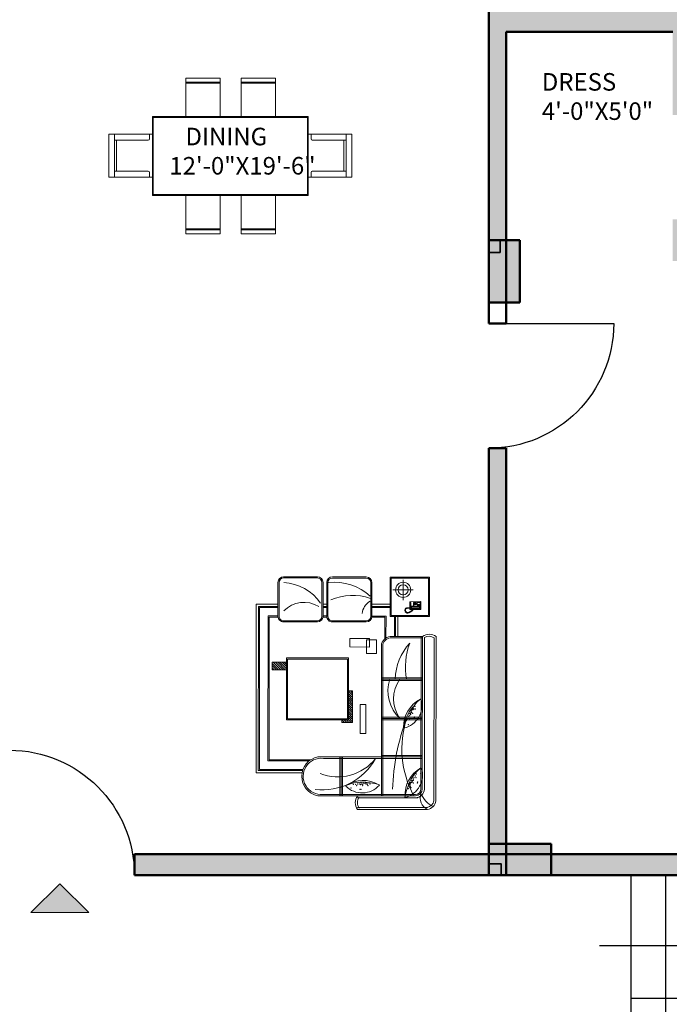
# Model space of a CAD drawing. Units: inches. Extents: x -7 to 1228, y -146 to 1091.
# Tile 82 of 88: x 816 to 1003, y 531 to 814. Entities that reach past the tile are written whole.
import ezdxf

# ---------------------------------------------------------------- set-up
doc = ezdxf.new("R2010")
doc.units = ezdxf.units.IN
for name, color, linetype, lineweight in [('A-ANNO-SYMB', 30, 'Continuous', 18), ('A-AREA-IDEN', 7, 'Continuous', 18), ('A-COLS', 6, 'Continuous', 35), ('A-DOOR', 4, 'Continuous', 25), ('A-FLOR-STRS', 1, 'Continuous', 25), ('A-FURN', 8, 'Continuous', 18), ('A-WALL', 7, 'Continuous', 50), ('A-WALL-PATT', 251, 'Continuous', 13)]:
    doc.layers.add(name, color=color, linetype=linetype, lineweight=lineweight)
doc.styles.get("Standard").update_dxf_attribs({"font": 'arial.ttf'})

# ---------------------------------------------------------------- blocks, each defined once
blk = doc.blocks.new('A$C317A697B')
for p, q in [((-116, 441), (-514, 441)), ((-514, 441), (-514, 0)), ((-116, 398), (-514, 398)), ((-116, 385), (-514, 385)), ((-116, 0), (-116, 441)), ((523, 441), (125, 441)), ((125, 441), (125, 0)), ((523, 398), (125, 398)), ((523, 385), (125, 385)), ((523, 0), (523, 441)), ((-899, -912), (-899, 0)), ((-899, 0), (899, 0)), ((899, 0), (899, -912)), ((-889, -902), (-889, -10)), ((-889, -10), (889, -10)), ((889, -10), (889, -902)), ((-899, -205), (-1402, -205)), ((-1402, -205), (-1402, -699)), ((-1336, -205), (-1336, -699)), ((-932, -205), (-932, -259)), ((899, -205), (1402, -205)), ((932, -205), (932, -259)), ((1336, -205), (1336, -699)), ((1402, -205), (1402, -699)), ((-946, -274), (-1336, -274)), ((-1311, -274), (-1311, -630)), ((946, -274), (1336, -274)), ((1311, -274), (1311, -630)), ((-946, -630), (-1336, -630)), ((-932, -699), (-932, -645)), ((932, -699), (932, -645)), ((946, -630), (1336, -630)), ((-1402, -699), (-899, -699)), ((1402, -699), (899, -699)), ((889, -902), (-889, -902)), ((899, -912), (-899, -912)), ((-514, -1353), (-514, -912)), ((-116, -912), (-116, -1353)), ((125, -1353), (125, -912)), ((523, -912), (523, -1353)), ((-116, -1297), (-514, -1297)), ((-116, -1309), (-514, -1309)), ((-116, -1353), (-514, -1353)), ((523, -1297), (125, -1297)), ((523, -1309), (125, -1309)), ((523, -1353), (125, -1353))]:
    blk.add_line(p, q)
for centre, start, end in [((-946, -259), 270, 0), ((946, -259), 180, 270), ((-946, -645), 0, 90), ((946, -645), 90, 180)]:
    blk.add_arc(centre, 14.7, start, end)
blk = doc.blocks.new('A$C327A19D4')
for p, q in [((1059, 3191), (3976, 3191)), ((1078, 3155), (3976, 3155)), ((703, 3073), (3, 3073)), ((3, 3073), (3, 2373)), ((683, 3053), (23, 3053)), ((23, 3053), (23, 2393)), ((683, 2393), (683, 3053)), ((703, 2373), (703, 3073)), ((1076, 2985), (3780, 2985)), ((4090, 3043), (4090, 1800)), ((4126, 3043), (4126, 1800)), ((1056, 2949), (3763, 2949)), ((1056, 2403), (1056, 2949)), ((1056, 2925), (3763, 2925)), ((1080, 2403), (1080, 2949)), ((1791, 2223), (1791, 2949)), ((1815, 2465), (1815, 2949)), ((1815, 2223), (1815, 2872)), ((1815, 2223), (1815, 2872)), ((1815, 2465), (1815, 2872)), ((1815, 2465), (1815, 2872)), ((1839, 2223), (1839, 2949)), ((2487, 2223), (2487, 2949)), ((2511, 2223), (2511, 2949)), ((2535, 2223), (2535, 2949)), ((3169, 2223), (3169, 2949)), ((3193, 2465), (3193, 2949)), ((3193, 2223), (3193, 2872)), ((3193, 2223), (3193, 2872)), ((3193, 2465), (3193, 2872)), ((3193, 2465), (3193, 2872)), ((3221, 1195), (3221, 2949)), ((3860, 2828), (3860, 1185)), ((3884, 2828), (3884, 1095)), ((3920, 2867), (3920, 1802)), ((231, 2784), (227, 2425)), ((49, 2607), (409, 2603)), ((703, 2512), (1056, 2512)), ((703, 2472), (1056, 2472)), ((703, 2452), (1056, 2452)), ((3, 2373), (703, 2373)), ((23, 2393), (683, 2393)), ((484, 2052), (484, 2373)), ((524, 2052), (524, 2373)), ((544, 2052), (544, 2373)), ((694, 2052), (694, 2302)), ((694, 2302), (1084, 2302)), ((714, 2051), (714, 2282)), ((714, 2282), (1098, 2282)), ((1119, 2135), (1357, 2135)), ((1119, 1958), (1119, 2135)), ((3884, 2247), (1184, 2247)), ((3884, 2223), (1184, 2223)), ((1357, 2135), (1357, 1958)), ((3195, 2235), (3195, 1095)), ((1092, 2007), (1244, 2007)), ((1092, 1659), (1092, 2007)), ((1357, 1958), (1119, 1958)), ((1244, 2007), (1244, 1659)), ((2265, 1945), (2780, 1945)), ((2265, 1845), (2265, 1945)), ((2780, 1945), (2780, 1845)), ((2780, 1845), (2265, 1845)), ((1244, 1659), (1092, 1659)), ((2539, 1638), (1439, 1638)), ((1439, 1638), (1439, 538)), ((2519, 1618), (1459, 1618)), ((1459, 1618), (1459, 558)), ((2023, 1638), (2023, 1711)), ((2023, 1711), (2585, 1711)), ((2519, 558), (2519, 1618)), ((2539, 538), (2539, 1638)), ((2585, 1711), (2585, 1522)), ((2585, 1522), (2539, 1522)), ((3884, 1532), (3195, 1532)), ((3884, 1508), (3195, 1508)), ((3884, 1484), (3195, 1484)), ((484, 1185), (484, 1252)), ((524, 1185), (524, 1252)), ((544, 1185), (544, 1252)), ((694, 1185), (694, 1252)), ((714, 1184), (714, 1253)), ((3247, 967), (3247, 230)), ((3267, 940), (3267, 210)), ((3417, 832), (3417, 60)), ((3437, 825), (3437, 40)), ((3477, 816), (3477, 0)), ((1439, 538), (2539, 538)), ((1459, 558), (2519, 558)), ((1516, 538), (1651, 538)), ((1516, 285), (1516, 538)), ((1651, 538), (1651, 285)), ((484, 0), (484, 385)), ((524, 40), (524, 385)), ((544, 60), (544, 385)), ((694, 210), (694, 385)), ((714, 230), (714, 386)), ((3267, 210), (694, 210)), ((3247, 230), (714, 230)), ((1651, 285), (1516, 285)), ((3437, 40), (524, 40)), ((3417, 60), (544, 60)), ((3477, 0), (484, 0))]:
    blk.add_line(p, q)
at = {"linetype": 'ByBlock'}
for p, q in [((438, 2915), (440, 2918)), ((439, 2728), (438, 2915)), ((440, 2918), (576, 2919)), ((451, 2906), (490, 2906)), ((451, 2856), (451, 2906)), ((491, 2856), (451, 2856)), ((453, 2831), (453, 2839)), ((453, 2839), (461, 2839)), ((461, 2831), (453, 2831)), ((453, 2824), (461, 2825)), ((453, 2816), (453, 2824)), ((461, 2816), (453, 2816)), ((453, 2801), (453, 2810)), ((453, 2810), (461, 2810)), ((461, 2802), (453, 2801)), ((461, 2839), (461, 2831)), ((461, 2825), (461, 2816)), ((461, 2810), (461, 2802)), ((466, 2839), (475, 2840)), ((467, 2831), (466, 2839)), ((475, 2831), (467, 2831)), ((467, 2816), (467, 2825)), ((467, 2825), (475, 2825)), ((475, 2817), (467, 2816)), ((467, 2802), (467, 2810)), ((467, 2810), (475, 2810)), ((475, 2802), (467, 2802)), ((475, 2840), (475, 2831)), ((475, 2825), (475, 2817)), ((475, 2810), (475, 2802)), ((480, 2840), (488, 2840)), ((480, 2831), (480, 2840)), ((488, 2832), (480, 2831)), ((480, 2817), (480, 2825)), ((480, 2825), (488, 2825)), ((488, 2817), (480, 2817)), ((480, 2810), (488, 2810)), ((480, 2802), (480, 2810)), ((488, 2802), (480, 2802)), ((488, 2840), (488, 2832)), ((488, 2825), (488, 2817)), ((488, 2810), (488, 2802)), ((490, 2906), (491, 2856)), ((505, 2903), (494, 2903)), ((494, 2903), (494, 2899)), ((494, 2899), (505, 2899)), ((495, 2895), (495, 2891)), ((505, 2895), (495, 2895)), ((495, 2891), (505, 2891)), ((495, 2887), (495, 2883)), ((505, 2887), (495, 2887)), ((495, 2883), (505, 2883)), ((495, 2879), (495, 2875)), ((505, 2879), (495, 2879)), ((495, 2875), (505, 2875)), ((495, 2871), (495, 2867)), ((506, 2871), (495, 2871)), ((495, 2867), (506, 2867)), ((495, 2863), (495, 2859)), ((506, 2863), (495, 2863)), ((495, 2859), (506, 2859)), ((505, 2899), (505, 2903)), ((505, 2891), (505, 2895)), ((505, 2883), (505, 2887)), ((505, 2875), (505, 2879)), ((506, 2867), (506, 2871)), ((506, 2859), (506, 2863)), ((515, 2908), (520, 2914)), ((516, 2744), (515, 2908)), ((520, 2910), (519, 2905)), ((519, 2905), (531, 2893)), ((519, 2905), (519, 2868)), ((519, 2868), (522, 2862)), ((520, 2914), (561, 2915)), ((526, 2913), (520, 2910)), ((522, 2862), (526, 2855)), ((522, 2790), (526, 2797)), ((532, 2895), (526, 2913)), ((526, 2913), (558, 2913)), ((526, 2855), (527, 2845)), ((526, 2797), (528, 2806)), ((527, 2845), (527, 2832)), ((528, 2806), (527, 2832)), ((531, 2893), (532, 2895)), ((532, 2832), (531, 2893)), ((551, 2896), (532, 2895)), ((532, 2832), (532, 2759)), ((551, 2896), (558, 2913)), ((553, 2893), (551, 2896)), ((565, 2905), (553, 2893)), ((553, 2832), (553, 2893)), ((553, 2832), (554, 2759)), ((558, 2855), (557, 2846)), ((557, 2846), (557, 2832)), ((557, 2806), (557, 2832)), ((559, 2797), (557, 2806)), ((558, 2913), (563, 2911)), ((562, 2862), (558, 2855)), ((563, 2790), (559, 2797)), ((561, 2915), (568, 2908)), ((565, 2869), (562, 2862)), ((563, 2911), (565, 2905)), ((565, 2905), (565, 2869)), ((568, 2908), (569, 2745)), ((576, 2919), (578, 2916)), ((578, 2916), (580, 2729)), ((442, 2726), (439, 2728)), ((543, 2726), (442, 2726)), ((453, 2787), (453, 2795)), ((453, 2795), (461, 2795)), ((461, 2787), (453, 2787)), ((468, 2743), (455, 2743)), ((455, 2743), (455, 2735)), ((455, 2735), (469, 2735)), ((461, 2795), (461, 2787)), ((467, 2787), (467, 2795)), ((467, 2795), (475, 2795)), ((475, 2787), (467, 2787)), ((469, 2735), (468, 2743)), ((487, 2743), (474, 2743)), ((474, 2743), (474, 2735)), ((474, 2735), (487, 2735)), ((475, 2795), (475, 2787)), ((480, 2787), (480, 2795)), ((480, 2795), (488, 2795)), ((488, 2787), (480, 2787)), ((487, 2735), (487, 2743)), ((488, 2795), (488, 2787)), ((493, 2744), (493, 2735)), ((506, 2744), (493, 2744)), ((493, 2735), (506, 2735)), ((497, 2795), (507, 2795)), ((497, 2787), (497, 2795)), ((507, 2787), (497, 2787)), ((506, 2735), (506, 2744)), ((507, 2795), (507, 2787)), ((523, 2737), (516, 2744)), ((520, 2783), (522, 2790)), ((520, 2746), (520, 2783)), ((520, 2746), (532, 2759)), ((521, 2741), (520, 2746)), ((527, 2738), (521, 2741)), ((542, 2737), (523, 2737)), ((533, 2756), (527, 2738)), ((527, 2738), (542, 2738)), ((532, 2759), (533, 2756)), ((552, 2756), (533, 2756)), ((546, 2743), (542, 2743)), ((542, 2743), (542, 2731)), ((542, 2731), (545, 2717)), ((545, 2717), (549, 2704)), ((547, 2732), (546, 2743)), ((546, 2738), (559, 2739)), ((562, 2737), (546, 2737)), ((549, 2696), (546, 2692)), ((546, 2692), (546, 2686)), ((546, 2686), (554, 2685)), ((554, 2685), (546, 2680)), ((546, 2680), (547, 2672)), ((548, 2723), (547, 2732)), ((547, 2672), (555, 2672)), ((577, 2726), (548, 2726)), ((552, 2710), (548, 2723)), ((549, 2704), (548, 2697)), ((548, 2697), (549, 2696)), ((555, 2672), (548, 2666)), ((548, 2666), (551, 2659)), ((551, 2659), (560, 2661)), ((554, 2759), (552, 2756)), ((552, 2756), (559, 2739)), ((553, 2703), (552, 2710)), ((552, 2696), (553, 2703)), ((557, 2693), (552, 2696)), ((566, 2747), (554, 2759)), ((556, 2687), (557, 2693)), ((558, 2669), (556, 2687)), ((560, 2661), (556, 2653)), ((556, 2653), (560, 2648)), ((568, 2656), (558, 2669)), ((559, 2739), (565, 2741)), ((560, 2648), (566, 2653)), ((569, 2745), (562, 2737)), ((566, 2783), (563, 2790)), ((565, 2741), (566, 2747)), ((566, 2653), (565, 2646)), ((565, 2646), (570, 2642)), ((566, 2747), (566, 2783)), ((583, 2649), (568, 2656)), ((570, 2642), (577, 2648)), ((577, 2648), (576, 2639)), ((576, 2639), (582, 2637)), ((580, 2729), (577, 2726)), ((587, 2779), (579, 2779)), ((579, 2775), (584, 2774)), ((582, 2637), (585, 2645)), ((599, 2647), (583, 2649)), ((584, 2774), (587, 2772)), ((585, 2645), (589, 2637)), ((590, 2777), (587, 2779)), ((587, 2772), (591, 2770)), ((589, 2637), (593, 2637)), ((594, 2771), (590, 2777)), ((591, 2770), (593, 2768)), ((595, 2768), (592, 2765)), ((592, 2765), (597, 2757)), ((593, 2768), (595, 2768)), ((593, 2637), (595, 2645)), ((599, 2771), (594, 2771)), ((595, 2645), (598, 2636)), ((597, 2757), (606, 2742)), ((598, 2636), (604, 2637)), ((602, 2770), (599, 2771)), ((599, 2760), (603, 2767)), ((606, 2763), (599, 2760)), ((615, 2654), (599, 2647)), ((603, 2767), (602, 2770)), ((604, 2750), (608, 2758)), ((612, 2753), (604, 2750)), ((604, 2645), (610, 2639)), ((604, 2637), (604, 2645)), ((608, 2758), (606, 2763)), ((606, 2742), (612, 2731)), ((608, 2742), (614, 2749)), ((615, 2746), (608, 2742)), ((610, 2639), (615, 2642)), ((614, 2749), (612, 2753)), ((612, 2731), (614, 2730)), ((613, 2733), (618, 2740)), ((621, 2736), (613, 2733)), ((614, 2730), (613, 2728)), ((613, 2728), (622, 2712)), ((614, 2650), (619, 2643)), ((615, 2642), (614, 2650)), ((618, 2740), (615, 2746)), ((627, 2666), (615, 2654)), ((619, 2643), (624, 2647)), ((620, 2723), (624, 2730)), ((627, 2725), (620, 2723)), ((620, 2654), (628, 2651)), ((624, 2647), (620, 2654)), ((624, 2730), (621, 2736)), ((622, 2712), (631, 2687)), ((626, 2712), (630, 2720)), ((634, 2713), (626, 2712)), ((630, 2720), (627, 2725)), ((631, 2687), (627, 2666)), ((628, 2702), (636, 2705)), ((637, 2702), (628, 2702)), ((628, 2661), (636, 2659)), ((632, 2654), (628, 2661)), ((628, 2651), (632, 2654)), ((631, 2672), (640, 2672)), ((638, 2665), (631, 2672)), ((633, 2691), (639, 2696)), ((641, 2691), (633, 2691)), ((636, 2705), (634, 2713)), ((634, 2681), (642, 2684)), ((641, 2677), (634, 2681)), ((636, 2659), (638, 2665)), ((639, 2696), (637, 2702)), ((640, 2672), (641, 2677)), ((642, 2684), (641, 2691))]:
    blk.add_line(p, q, dxfattribs=at)
at = {"ltscale": 5}
for p, q in [((0, 1352), (0, 1952)), ((20, 1352), (20, 1952)), ((100, 2052), (700, 2052)), ((100, 2032), (700, 2032)), ((780, 1952), (780, 1352)), ((800, 1952), (800, 1352)), ((2023, 1673), (2061, 1711)), ((2027, 1638), (2100, 1711)), ((2067, 1638), (2139, 1711)), ((2106, 1638), (2179, 1711)), ((2145, 1638), (2218, 1711)), ((2184, 1638), (2257, 1711)), ((2224, 1638), (2296, 1711)), ((2263, 1638), (2336, 1711)), ((2302, 1638), (2375, 1711)), ((2341, 1638), (2414, 1711)), ((2381, 1638), (2453, 1711)), ((2420, 1638), (2493, 1711)), ((2459, 1638), (2532, 1711)), ((2498, 1638), (2571, 1711)), ((2538, 1638), (2585, 1685)), ((2539, 1601), (2585, 1646)), ((2539, 1561), (2585, 1607)), ((2539, 1522), (2585, 1568)), ((2578, 1522), (2585, 1528)), ((700, 1272), (100, 1272)), ((700, 1252), (100, 1252)), ((0, 485), (0, 1085)), ((20, 485), (20, 1085)), ((100, 1185), (700, 1185)), ((100, 1165), (700, 1165)), ((780, 1085), (780, 485)), ((800, 1085), (800, 485)), ((1516, 499), (1555, 538)), ((1516, 460), (1594, 538)), ((1516, 421), (1634, 538)), ((700, 405), (100, 405)), ((700, 385), (100, 385)), ((1516, 382), (1651, 516)), ((1516, 342), (1651, 477)), ((1516, 303), (1651, 438)), ((1537, 285), (1651, 398)), ((1576, 285), (1651, 359)), ((1616, 285), (1651, 320))]:
    blk.add_line(p, q, dxfattribs=at)
for radius in [134, 88.7]:
    blk.add_circle((229, 2605), radius)
for centre, radius, start, end in [((1218, 3068), 201, 142.4201, 216.3682), ((1218, 3068), 165, 148.4003, 210.2229), ((3943, 3007), 150, 10.9855, 79.893), ((3943, 3007), 187, 10.9855, 79.893), ((3763, 2828), 157, 0, 90), ((3657, 3353), 468, 293.6733, 332.9672), ((3921, 3138), 226, 250.4844, 335.1673), ((2545, 3192), 468, 214.7097, 257.8799), ((2283, 2531), 409, 13.4523, 105.9639), ((2657, 3163), 547, 207.1715, 271.8037), ((3869, 3188), 547, 208.8478, 273.48), ((3911, 3323), 657, 217.6007, 253.5739), ((3517, 2544), 409, 14.6876, 107.1992), ((3763, 2828), 121, 0, 90), ((3763, 2828), 96.8, 0, 90), ((1594, 3859), 1211, 249.7283, 280.5443), ((1853, 3485), 1021, 228.2765, 267.8541), ((2752, 3267), 657, 227.0776, 263.0508), ((3052, 4350), 1764, 252.1519, 298.1592), ((3865, 6197), 3777, 248.9971, 268.5461), ((3951, 3106), 468, 222.7716, 265.9418), ((2024, 3008), 670, 251.8392, 316.629), ((2163, 3036), 599, 234.5154, 305.4846), ((1243, 2401), 187, 179.2584, 251.6848), ((1243, 2401), 163, 179.2584, 251.6848), ((4159, 1898), 547, 149.1529, 213.7851), ((4124, 2008), 468, 156.691, 199.8613), ((3425, 1881), 409, 315.4337, 47.9453), ((4298, 1873), 657, 169.059, 205.0321), ((4007, 1962), 201, 232.4201, 306.3682), ((4007, 1962), 165, 232.4201, 306.3682)]:
    blk.add_arc(centre, radius, start, end)
at = {"ltscale": 20}
for centre, radius, start, end in [((2701, 1449), 849, 338.2682, 52.2695), ((2703, 1175), 1078, 353.1988, 61.2564), ((3540, 1161), 351, 190.8398, 349.1602), ((3540, 1156), 321, 172.9078, 5.2194)]:
    blk.add_arc(centre, radius, start, end, dxfattribs=at)
at = {"ltscale": 5}
for centre, radius, start, end in [((100, 1952), 100, 90, 180), ((100, 1952), 80, 90, 180), ((1024, 1388), 928, 137.1341, 186.5635), ((1307, 1706), 979, 160.9364, 203.1944), ((676, 2156), 279, 209.1633, 264.4137), ((700, 1952), 100, 0, 90), ((700, 1952), 80, 0, 90), ((100, 1352), 100, 180, 270), ((100, 1352), 80, 180, 270), ((700, 1352), 80, 270, 0), ((700, 1352), 100, 270, 0), ((100, 1085), 100, 90, 180), ((100, 1085), 80, 90, 180), ((968, 436), 868, 125.4807, 176.5616), ((949, 846), 497, 147.8484, 226.1244), ((700, 1085), 100, 0, 90), ((700, 1085), 80, 0, 90), ((100, 485), 100, 180, 270), ((100, 485), 80, 180, 270), ((700, 485), 100, 270, 0), ((700, 485), 80, 270, 0)]:
    blk.add_arc(centre, radius, start, end, dxfattribs=at)
for p in [(2298, 2818), (2344, 2802), (2345, 2825), (2485, 2814), (2498, 2803), (3492, 2920), (3495, 2842), (3535, 2825), (3560, 2838), (3561, 2800), (3641, 2868), (3657, 2862), (2329, 2780), (2356, 2781), (2375, 2736), (2410, 2757), (2421, 2774), (2421, 2720), (2444, 2738), (2445, 2691), (2459, 2715), (2481, 2700), (2514, 2718), (2515, 2690), (2551, 2664), (2620, 2701), (3571, 2765), (3585, 2789), (3609, 2758), (3612, 2788), (3646, 2728), (3647, 2768), (3655, 2787), (3694, 2735), (3707, 2710), (3719, 2734), (3738, 2747), (3756, 2703), (3660, 1974), (3676, 1951), (3677, 2020), (3687, 1973), (3707, 1984), (3646, 1828), (3648, 1911), (3658, 1864), (3673, 1803), (3674, 1829), (3683, 1768), (3684, 1893), (3686, 1853), (3705, 1892), (3706, 1784), (3770, 1842), (3772, 1859), (3680, 1724), (3748, 1685)]:
    blk.add_point(p)
blk = doc.blocks.new('DOOR-900')
blk.add_line((36, 0), (36, 36))
blk.add_arc((36, 0), 36, 90, 180)

msp = doc.modelspace()

# ---------------------------------------------------------------- hatches: boundary and pattern name
at = {"layer": 'A-ANNO-SYMB'}
h = msp.add_hatch(color=256, dxfattribs=at)
h.dxf.hatch_style = 1
h.paths.add_polyline_path([(827.53, 565.53), (819.19, 557.2), (835.87, 557.2)])
at = {"layer": 'A-COLS'}
h = msp.add_hatch(color=256, dxfattribs=at)
h.dxf.hatch_style = 1
h.paths.add_polyline_path([(951, 733), (960, 733), (960, 751), (954.29, 751), (954.29, 747.45), (951, 747.45)])
h = msp.add_hatch(color=256, dxfattribs=at)
h.dxf.hatch_style = 1
h.paths.add_polyline_path([(954.29, 747.45), (954.29, 751), (951, 751), (951, 747.45)])
h = msp.add_hatch(color=256, dxfattribs=at)
h.dxf.hatch_style = 1
h.paths.add_polyline_path([(969, 568), (969, 577), (951, 577), (951, 571.29), (954.55, 571.29), (954.55, 568)])
h = msp.add_hatch(color=256, dxfattribs=at)
h.dxf.hatch_style = 1
h.paths.add_polyline_path([(954.55, 571.29), (951, 571.29), (951, 568), (954.55, 568)])
at = {"layer": 'A-WALL-PATT'}
h = msp.add_hatch(color=256, dxfattribs=at)
h.dxf.hatch_style = 1
h.paths.add_polyline_path([(69, 568), (60, 568), (60, 493), (63.29, 493), (69, 493)])
h.paths.add_polyline_path([(69, 662.41), (60, 662.41), (60, 586), (69, 586)], flags=17)
h.paths.add_polyline_path([(69, 723), (184, 723), (184, 734), (179, 734), (179, 728), (69, 728), (69, 741.62), (60, 741.62), (60, 698.41), (69, 698.41)], flags=17)
h.paths.add_polyline_path([(69, 782), (231, 782), (231, 728), (231, 723), (231, 586), (236, 586), (236, 787), (69, 787), (69, 800.13), (60, 800.13), (60, 765.62), (69, 765.62)])
h.paths.add_polyline_path([(184, 842), (189, 842), (189, 848), (173, 848), (173, 842), (179, 842), (179, 787), (184, 787)])
h.paths.add_polyline_path([(118.22, 69), (69, 69), (69, 60), (118.22, 60)])
h.paths.add_polyline_path([(227, 69), (154.22, 69), (154.22, 60), (227, 60)])
h.paths.add_polyline_path([(236, 60), (232.71, 60), (227, 60), (227, 36), (236, 36)])
h.paths.add_polyline_path([(389, 60), (380, 60), (380, 36), (389, 36)])
h.paths.add_polyline_path([(384, 181), (380, 181), (380, 115), (380, 78), (384, 78)])
h.paths.add_polyline_path([(380, 115), (334.55, 115), (334.55, 109), (380, 109)])
h.paths.add_polyline_path([(274.55, 115), (236, 115), (236, 201), (232.71, 201), (231, 201), (231, 78), (236, 78), (236, 109), (274.55, 109)])
h.paths.add_polyline_path([(69, 123), (60, 123), (60, 78), (69, 78)])
h.paths.add_polyline_path([(69, 201), (60, 201), (60, 159), (69, 159)])
h.paths.add_polyline_path([(143, 219), (69, 219), (69, 213), (143, 213)], flags=17)
h.paths.add_polyline_path([(189, 219), (184, 219), (184, 274), (231, 274), (231, 219), (236, 219), (236, 279), (184, 279), (184, 297), (179, 297), (179, 279), (69, 279), (69, 290.91), (60, 290.91), (60, 262.18), (69, 262.18), (69, 274), (179, 274), (179, 219), (173, 219), (173, 213), (189, 213)])
h.paths.add_polyline_path([(69, 238.18), (60, 238.18), (60, 219), (69, 219)], flags=17)
h.paths.add_polyline_path([(69, 333), (60, 333), (60, 314.91), (69, 314.91), (69, 316.96)])
h.paths.add_polyline_path([(190, 338), (184, 338), (69, 338), (69, 333), (179, 333), (179, 327), (184, 327), (184, 333.02), (190, 333.05)])
h.paths.add_polyline_path([(69, 386.81), (60, 386.81), (60, 351), (69, 351)])
h.paths.add_polyline_path([(69, 475), (60, 475), (60, 422.81), (69, 422.81)])
h.paths.add_polyline_path([(236, 475), (231, 475), (231, 351.24), (236, 351.24)])
h.paths.add_polyline_path([(384, 475), (380, 475), (380, 362), (384, 362)])
h.paths.add_polyline_path([(547, 307), (439, 307), (439, 356), (445, 356), (445, 362), (433, 362), (433, 307), (380, 307), (380, 244), (380, 241), (384, 241), (384, 301), (433, 301), (433, 277), (439, 277), (439, 301), (547, 301)])
h.paths.add_polyline_path([(547, 241), (439, 241), (439, 247), (433, 247), (433, 235), (547, 235)])
h.paths.add_polyline_path([(450, 69), (440.29, 69), (424.89, 69), (389, 69), (389, 60), (450, 60)])
h.paths.add_polyline_path([(547, 69), (486, 69), (486, 60), (547, 60)])
h.paths.add_polyline_path([(556, 148.27), (547, 148.27), (547, 78), (556, 78)])
h.paths.add_polyline_path([(556, 223), (547, 223), (547, 195), (547, 184.27), (556, 184.27)])
h.paths.add_polyline_path([(556, 311.19), (547, 311.19), (547, 273.08), (556, 273.08)])
h.paths.add_polyline_path([(556, 344), (552.71, 344), (547, 344), (547, 335.19), (556, 335.19)])
h.paths.add_polyline_path([(556, 249.08), (547, 249.08), (547, 241), (556, 241)])
h.paths.add_polyline_path([(547, 362), (475, 362), (475, 356), (547, 356)], flags=0)
h.paths.add_polyline_path([(556, 399.62), (547, 399.62), (547, 362), (556, 362)])
h.paths.add_polyline_path([(556, 475), (547, 475), (547, 435.62), (556, 435.62)])
h.paths.add_polyline_path([(547, 493), (389, 493), (389, 487), (547, 487)])
h.paths.add_polyline_path([(380, 493), (278, 493), (278, 487), (380, 487)])
h.paths.add_polyline_path([(227, 493), (69, 493), (69, 487), (227, 487)])
h.paths.add_polyline_path([(643, 122.44), (634, 122.44), (634, 78), (643, 78)])
h.paths.add_polyline_path([(702.5, 69), (692.79, 69), (677.39, 69), (643, 69), (643, 60), (702.5, 60)])
h.paths.add_polyline_path([(798, 69), (738.5, 69), (738.5, 60), (798, 60)])
h.paths.add_polyline_path([(807, 60), (803.71, 60), (798, 60), (798, 36), (807, 36)])
h.paths.add_polyline_path([(807, 109), (846.75, 109), (846.75, 115), (807, 115), (807, 159), (802, 159), (802, 78), (807, 78)])
h.paths.add_polyline_path([(807, 201), (802, 201), (802, 195), (807, 195)])
h.paths.add_polyline_path([(643, 201), (634, 201), (634, 158.44), (643, 158.44)])
h.paths.add_polyline_path([(756, 225), (751, 225), (751, 219), (643, 219), (643, 213), (756, 213)])
h.paths.add_polyline_path([(643, 240.85), (634, 240.85), (634, 219), (643, 219)])
h.paths.add_polyline_path([(643, 274), (643, 288.63), (634, 288.63), (634, 264.85), (643, 264.85)])
h.paths.add_polyline_path([(802, 279), (756, 279), (756, 297), (751, 297), (751, 279), (643, 279), (643, 274), (751, 274), (751, 255), (756, 255), (756, 274), (802, 274)])
h.paths.add_polyline_path([(807, 333), (803.71, 333), (802, 333), (802, 279), (802, 274), (802, 219), (807, 219)])
h.paths.add_polyline_path([(956, 182), (951, 182), (951, 115), (906.75, 115), (906.75, 109), (951, 109), (951, 78), (956, 78)])
h.paths.add_polyline_path([(960, 60), (951, 60), (951, 36), (960, 36)])
h.paths.add_polyline_path([(1021, 69), (1005.78, 69), (960, 69), (960, 60), (1021, 60)])
h.paths.add_polyline_path([(956, 224), (951, 224), (951, 218), (956, 218)])
h.paths.add_polyline_path([(956, 302), (1004, 302), (1004, 278), (1010, 278), (1010, 302), (1118, 302), (1118, 290.81), (1127, 290.81), (1127, 326.97), (1118, 326.97), (1118, 320.97), (1118, 307), (1010, 307), (1010, 356), (1016, 356), (1016, 362), (1004, 362), (1004, 307), (951, 307), (951, 244), (951, 242), (954.29, 242), (956, 242)])
h.paths.add_polyline_path([(643, 333), (634, 333), (634, 312.63), (643, 312.63), (643, 316.96)])
h.paths.add_polyline_path([(756, 338), (643, 338), (643, 333), (751, 333), (751, 327), (756, 327)])
h.paths.add_polyline_path([(643, 388), (634, 388), (634, 351), (643, 351)])
h.paths.add_polyline_path([(807, 357), (802, 357), (802, 351), (807, 351)])
h.paths.add_polyline_path([(807, 475), (802, 475), (802, 393), (807, 393)])
h.paths.add_polyline_path([(643, 475), (634, 475), (634, 424), (643, 424)])
h.paths.add_polyline_path([(798, 493), (643, 493), (643, 487), (798, 487)])
h.paths.add_polyline_path([(634, 493), (556, 493), (556, 487), (634, 487)])
h.paths.add_polyline_path([(813, 493), (807, 493), (807, 487), (813, 487)])
h.paths.add_polyline_path([(951, 493), (849, 493), (849, 487), (951, 487)])
h.paths.add_polyline_path([(956, 484), (951, 484), (951, 374), (956, 374)])
h.paths.add_polyline_path([(1109, 493), (969, 493), (969, 487), (1109, 487)])
h.paths.add_polyline_path([(1127, 484), (1118, 484), (1118, 450.64), (1127, 450.64)])
h.paths.add_polyline_path([(1127, 414.64), (1118, 414.64), (1118, 365), (1127, 365)])
h.paths.add_polyline_path([(1109, 362), (1046, 362), (1046, 356), (1109, 356)], flags=17)
h.paths.add_polyline_path([(1127, 356), (1123.45, 356), (1118, 356), (1118, 350.97), (1127, 350.97)], flags=0)
h.paths.add_polyline_path([(1127, 266.81), (1118, 266.81), (1118, 262.36), (1118, 242), (1127, 242)], flags=17)
h.paths.add_polyline_path([(1118, 242), (1010, 242), (1010, 248), (1004, 248), (1004, 237), (1118, 237)])
h.paths.add_polyline_path([(1127, 224), (1118, 224), (1118, 170), (1127, 170)])
h.paths.add_polyline_path([(1127, 134), (1118, 134), (1118, 78), (1127, 78)])
h.paths.add_polyline_path([(1118, 69), (1057, 69), (1057, 60), (1118, 60)])
h.paths.add_polyline_path([(227, 571.55), (227, 574), (69, 574), (69, 568), (227, 568)])
h.paths.add_polyline_path([(380, 571.55), (380, 574), (278, 574), (278, 568), (380, 568)])
h.paths.add_polyline_path([(242, 574), (236, 574), (236, 568), (242, 568)])
h.paths.add_polyline_path([(547, 571.55), (547, 574), (389, 574), (389, 568), (547, 568)])
h.paths.add_polyline_path([(384, 733), (380, 733), (380, 586), (384, 586)])
h.paths.add_polyline_path([(556, 646), (634, 646), (634, 655), (547, 655), (547, 586), (556, 586)])
h.paths.add_polyline_path([(634, 574), (556, 574), (556, 568), (634, 568)])
h.paths.add_polyline_path([(643, 655), (634, 655), (634, 586), (643, 586)])
h.paths.add_polyline_path([(798, 574), (643, 574), (643, 568), (798, 568)])
h.paths.add_polyline_path([(643, 663.85), (634, 663.85), (634, 655), (643, 655)])
h.paths.add_polyline_path([(556, 676.97), (547, 676.97), (547, 655), (556, 655)])
h.paths.add_polyline_path([(556, 733), (547, 733), (547, 712.97), (556, 712.97)])
h.paths.add_polyline_path([(643, 710), (634, 710), (634, 699.85), (643, 699.85)])
h.paths.add_polyline_path([(807, 668), (802, 668), (802, 586), (807, 586)])
h.paths.add_polyline_path([(951, 574), (849, 574), (849, 568), (951, 568)])
h.paths.add_polyline_path([(956, 691), (951, 691), (951, 577), (956, 577)])
h.paths.add_polyline_path([(1109, 574), (969, 574), (969, 568), (1109, 568)])
h.paths.add_polyline_path([(1127, 643.4), (1118, 643.4), (1118, 577), (1127, 577)])
h.paths.add_polyline_path([(1127, 568), (1123.45, 568), (1118, 568), (1118, 493), (1127, 493)])
h.paths.add_polyline_path([(1127, 733), (1118, 733), (1118, 679.4), (1127, 679.4)])
h.paths.add_polyline_path([(1127, 777.35), (1118, 777.35), (1118, 770.04), (1118, 751), (1127, 751)], flags=17)
h.paths.add_polyline_path([(1118, 751), (1010, 751), (1010, 757), (1004, 757), (1004, 745), (1118, 745)])
h.paths.add_polyline_path([(956, 811), (1004, 811), (1004, 787), (1010, 787), (1010, 811), (1017.87, 811), (1017.87, 811.63, -0.414214), (1018.25, 812), (1031.98, 812, -0.414214), (1032.35, 811.63), (1032.35, 811), (1118, 811), (1118, 801.35), (1127, 801.35), (1127, 834.69), (1118, 834.69), (1118, 830.24), (1118, 817), (1010, 817), (1010, 866), (1016, 866), (1016, 872), (1004, 872), (1004, 817), (956, 817), (956, 866), (951, 866), (951, 751), (954.29, 751), (956, 751)])
h.paths.add_polyline_path([(1118, 872), (1046, 872), (1046, 866), (1118, 866)], flags=17)
h.paths.add_polyline_path([(1127, 924.71), (1118, 924.71), (1118, 884), (1127, 884)])
h.paths.add_polyline_path([(1127, 866), (1123.71, 866), (1118, 866), (1118, 858.69), (1127, 858.69)], flags=17)
h.paths.add_polyline_path([(956, 983), (951, 983), (951, 952), (807, 952), (807, 983), (802, 983), (802, 902), (807, 902), (807, 946), (951, 946), (951, 884), (956, 884)])
h.paths.add_polyline_path([(807, 842), (802, 842), (802, 787), (756, 787), (756, 806), (751, 806), (751, 787), (643, 787), (643, 782), (751, 782), (751, 764), (756, 764), (756, 782), (802, 782), (802, 728), (807, 728)])
h.paths.add_polyline_path([(756, 848), (643, 848), (643, 842), (751, 842), (751, 836), (756, 836)])
h.paths.add_polyline_path([(756, 734), (751, 734), (751, 728), (643, 728), (643, 723), (756, 723)])
h.paths.add_polyline_path([(643, 749.79), (634, 749.79), (634, 728), (637.29, 728), (643, 728)])
h.paths.add_polyline_path([(643, 805.41), (634, 805.41), (634, 773.79), (643, 773.79)])
h.paths.add_polyline_path([(643, 896.66), (634, 896.66), (634, 860), (637.29, 860), (643, 860)])
h.paths.add_polyline_path([(643, 842), (634, 842), (634, 829.41), (643, 829.41)])
h.paths.add_polyline_path([(643, 983), (634, 983), (634, 932.66), (643, 932.66)])
h.paths.add_polyline_path([(1127, 983), (1118, 983), (1118, 960.71), (1127, 960.71)])
h.paths.add_polyline_path([(1118, 1001), (1077.53, 1001), (1077.53, 992), (1118, 992)])
h.paths.add_polyline_path([(1041.53, 1001), (960, 1001), (960, 992), (1041.53, 992)])
h.paths.add_polyline_path([(960, 1025), (951, 1025), (951, 1001), (954.29, 1001), (960, 1001)])
h.paths.add_polyline_path([(807, 1025), (798, 1025), (798, 1001), (807, 1001)])
h.paths.add_polyline_path([(798, 1001), (738.5, 1001), (738.5, 992), (798, 992)])
h.paths.add_polyline_path([(702.5, 1001), (643, 1001), (643, 992), (702.5, 992)])
h.paths.add_polyline_path([(547, 1001), (499.11, 1001), (499.11, 992), (547, 992)])
h.paths.add_polyline_path([(463.11, 1001), (389, 1001), (389, 992), (463.11, 992)])
h.paths.add_polyline_path([(389, 1025), (380, 1025), (380, 1022), (380, 1001), (383.29, 1001), (389, 1001)])
h.paths.add_polyline_path([(236, 1025), (227, 1025), (227, 1001), (236, 1001)])
h.paths.add_polyline_path([(236, 983), (231, 983), (231, 860), (236, 860)])
h.paths.add_polyline_path([(274.55, 952), (236, 952), (236, 946), (274.55, 946)])
h.paths.add_polyline_path([(380, 952), (334.55, 952), (334.55, 946), (380, 946)])
h.paths.add_polyline_path([(384, 983), (380, 983), (380, 884), (383.29, 884), (384, 884)])
h.paths.add_polyline_path([(227, 1001), (155.01, 1001), (155.01, 992), (162.87, 992), (227, 992)])
h.paths.add_polyline_path([(119.01, 1001), (69, 1001), (69, 992), (119.01, 992)])
h.paths.add_polyline_path([(69, 983), (60, 983), (60, 922.99), (69, 922.99)])
h.paths.add_polyline_path([(69, 886.99), (60, 886.99), (60, 860), (63.29, 860), (69, 860)])
h.paths.add_polyline_path([(143, 848), (69, 848), (69, 842), (143, 842)])

# ---------------------------------------------------------------- linework, layer by layer
at = {"layer": 'A-ANNO-SYMB'}
for p, q in [((827.53, 565.53), (819.19, 557.2)), ((827.53, 565.53), (835.87, 557.2)), ((819.19, 557.2), (835.87, 557.2))]:
    msp.add_line(p, q, dxfattribs=at)
at = {"layer": 'A-COLS'}
for points in [[(951, 751), (954.29, 751), (954.29, 747.45), (951, 747.45)], [(951, 568), (951, 571.29), (954.55, 571.29), (954.55, 568)]]:
    msp.add_lwpolyline(points, close=True, dxfattribs=at)
at = {"layer": 'A-FLOR-STRS'}
for p, q in [((992, 493), (992, 568)), ((1002, 493), (1002, 568)), ((982.86, 547.69), (1035.65, 547.69)), ((992, 532.5), (1082, 532.5))]:
    msp.add_line(p, q, dxfattribs=at)
at = {"layer": 'A-WALL'}
for p, q in [((951, 727), (951, 946)), ((951, 817), (951, 727)), ((1004, 811), (956, 811)), ((956, 811), (956, 727)), ((956, 727), (956, 811)), ((956, 751), (951, 751)), ((951, 751), (960, 751)), ((951, 733), (951, 751)), ((960, 751), (960, 733)), ((960, 733), (960, 739)), ((960, 733), (951, 733)), ((951, 733), (956, 733)), ((951, 727), (956, 727)), ((951, 568), (951, 691)), ((951, 691), (956, 691)), ((951, 691), (951, 568)), ((956, 568), (956, 691)), ((956, 691), (956, 568)), ((951, 568), (951, 577)), ((951, 577), (969, 577)), ((969, 577), (969, 568)), ((1127, 574), (849, 574)), ((849, 568), (849, 574)), ((1127, 568), (849, 568)), ((969, 568), (951, 568))]:
    msp.add_line(p, q, dxfattribs=at)

# ---------------------------------------------------------------- block references
at = {"layer": 'A-DOOR', "extrusion": (0, 0, -1), "zscale": -1, "rotation": 89.99999999999984}
msp.add_blockref('DOOR-900', (-951, 691), dxfattribs=at)
at = {"layer": 'A-DOOR', "extrusion": (0, 0, -1), "zscale": -1}
msp.add_blockref('DOOR-900', (-849, 568), dxfattribs=at)
at = {"layer": 'A-FURN', "xscale": 0.024965713951469, "yscale": 0.024965713951469, "zscale": 0.024965713951469}
msp.add_blockref('A$C317A697B', (876.61, 786.6), dxfattribs=at)
at = {"layer": 'A-FURN', "xscale": 0.016235792481004, "yscale": 0.016235792481004, "zscale": 0.016235792481004, "rotation": 269.9431658144944}
msp.add_blockref('A$C327A19D4', (884.08, 653.96), dxfattribs=at)

# ---------------------------------------------------------------- texts
at = {"layer": 'A-AREA-IDEN', "attachment_point": 1}
for s, insert, char_height in [('DRESS\\P4\'-0"X5\'0"', (966.3, 799.11), 5.057), ('   DINING\\P12\'-0"X19\'-6"', (859.07, 783.36), 5.0568)]:
    msp.add_mtext_dynamic_manual_height_columns(s, width=137.2821, gutter_width=25.28, heights=[0], dxfattribs=dict(at, insert=insert, char_height=char_height))

doc.saveas('drawing.dxf')
